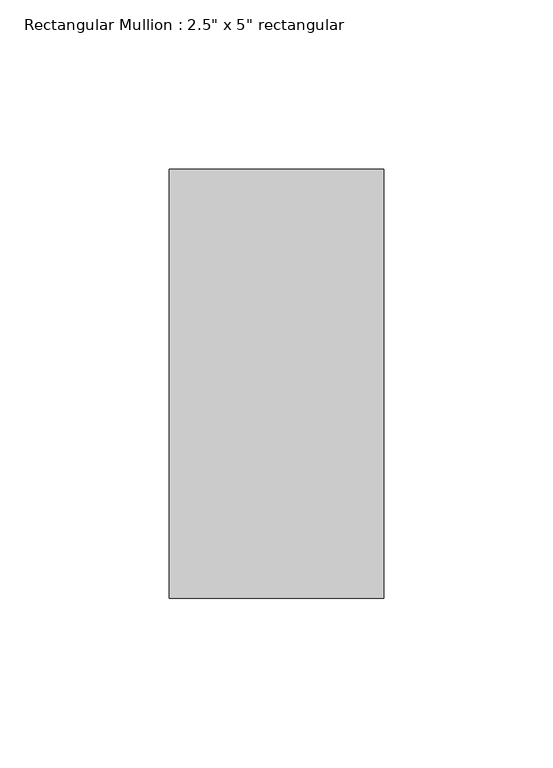
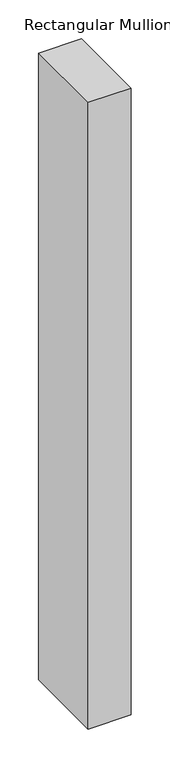
"""IFC4 building model written with IfcOpenShell, lengths in millimetres: member geometry."""

from ifc_helpers import new_model, si_unit, frame, origin, place, context, project, spatial, polyline, outline, extrude, source, transform, mapped, element, save


def member_fc2bd130(model_context):
    return source(origin(), model_context, "Body", "SweptSolid", [
        extrude(outline(polyline([(31.75, 63.5), (31.75, -63.5), (-31.75, -63.5), (-31.75, 63.5), (31.75, 63.5)])), frame((0.0, 0.0, -982.1333333), z_axis=(0.0, 0.0, 1.0), x_axis=(1.0, 0.0, 0.0)), (0.0, 0.0, 1.0), 982.1333333),
    ])


if __name__ == "__main__":
    model = new_model("IFC4")
    model_context = context("Model", 3, world=origin())
    ifc_project = project(units=[si_unit("LENGTHUNIT", "METRE", prefix="MILLI")], contexts=[model_context])
    site = spatial("IfcSite", under=ifc_project)
    building = spatial("IfcBuilding", under=site)
    placement = place(None, origin())
    member_shape = member_fc2bd130(model_context)
    element("IfcMember", 1, ObjectType="Rectangular Mullion : 2.5\" x 5\" rectangular", at=placement, inside=building, context=model_context, shape_type="MappedRepresentation", body=[
        mapped(member_shape, transform((0.0, 0.0, 0.0), x_axis=(1.0, 0.0, 0.0), y_axis=(0.0, 1.0, 0.0), z_axis=(0.0, 0.0, 1.0))),
    ])
    save(model, "model.ifc")

# Revit data of these elements
# Type "Rectangular Mullion : 2.5\" x 5\" rectangular"
#   built-in parameter 1007304 = 0.416667 (stored number, unit not read)
#   built-in parameter 1007301 = 0.104167 (stored number, unit not read)
#   built-in parameter 1007300 = 0.104167 (stored number, unit not read)
# Element 1 (IfcMember, "Rectangular Mullion : 2.5\" x 5\" rectangular")
#   Materials on its faces: "Aluminum"
# Materials
#   "Aluminum": class "Metal", colour RGB 247 247 247, transparency 0, Description = "Aluminum 6061", Cost = 0
